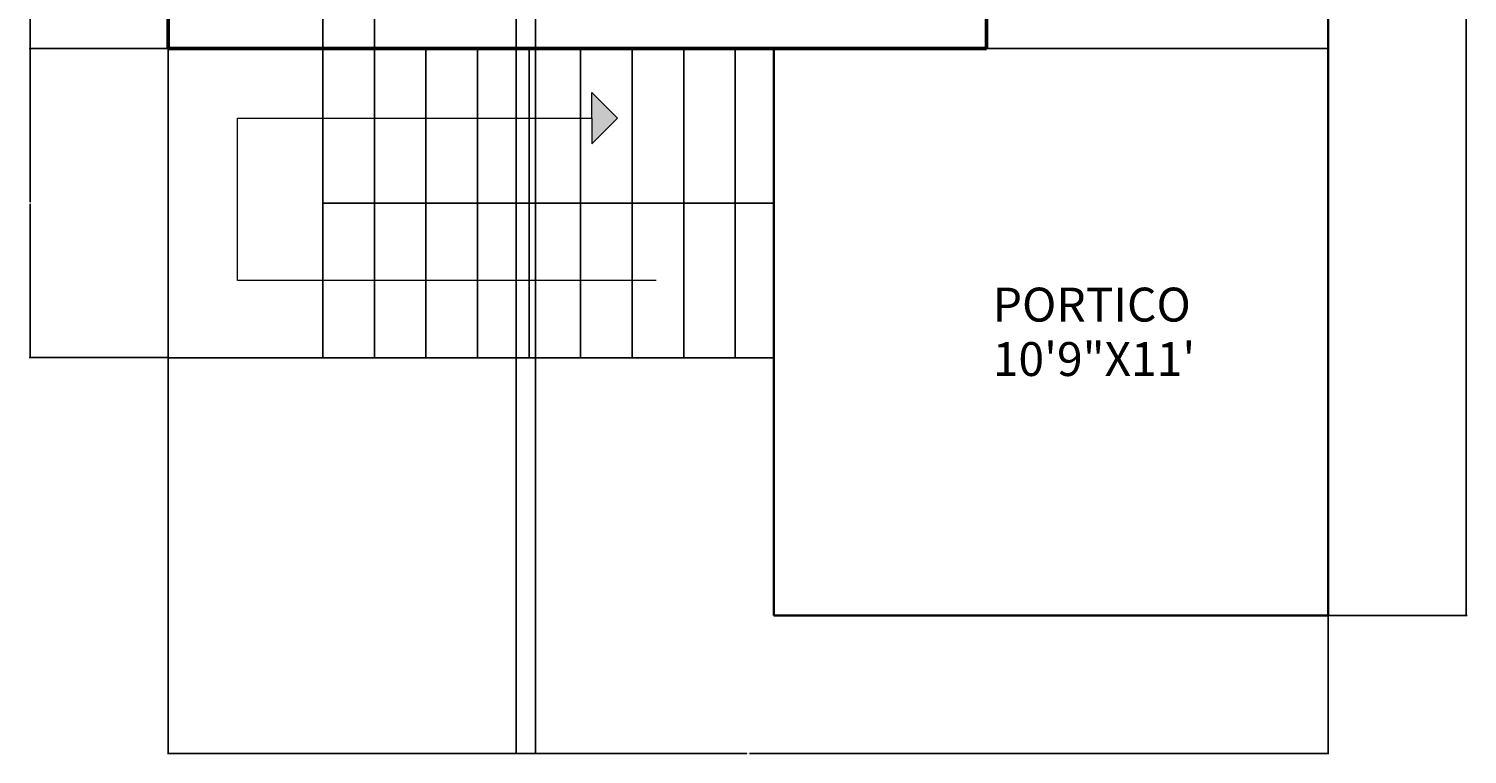
# Model space of a CAD drawing. Units: feet. Extents: x 1657 to 2001, y 1678 to 2367.
# Tile 1 of 4: x 1666 to 2001, y 1678 to 1847. Entities that reach past the tile are written whole.
import ezdxf

# ---------------------------------------------------------------- set-up
doc = ezdxf.new("R2010")
doc.units = ezdxf.units.FT
for name, color, linetype, lineweight in [('A-ANNO-DIMS', 2, 'Continuous', 18), ('A-ANNO-SYMB', 7, 'Continuous', 18), ('A-AREA-IDEN', 7, 'Continuous', 25), ('A-FLOR', 7, 'Continuous', 35), ('A-FLOR-STRS', 7, 'Continuous', 25), ('A-WALL', 7, 'Continuous', 50)]:
    doc.layers.add(name, color=color, linetype=linetype, lineweight=lineweight)
doc.styles.get("Standard").update_dxf_attribs({"font": 'arial.ttf'})
doc.dimstyles.get("Standard").update_dxf_attribs({"dimtxt": 0.18, "dimasz": 0.18, "dimexe": 0.18, "dimexo": 0.0625, "dimgap": 0.09, "dimtad": 0, "dimtih": 1, "dimtoh": 1, "dimdec": 4, "dimzin": 0, "dimdsep": 46, "dimtxsty": 'Standard', "dimcen": 0.09, "dimadec": 0, "dimazin": 0, "dimtfac": 1, "dimtdec": 4, "dimtofl": 0, "dimtmove": 0, "dimatfit": 3, "dimfxl": 1, "dimtolj": 1, "dimtzin": 0, "dimarcsym": 0})

# ---------------------------------------------------------------- blocks, each defined once
blk = doc.blocks.new('*D34')
at = {"layer": 'A-ANNO-DIMS', "color": 0, "lineweight": -2, "transparency": 16777216}
for p, q in [((1698.28, 1770.24), (1698.28, 1677.97)), ((1968.28, 1710.24), (1968.28, 1677.97)), ((1698.46, 1678.15), (1832.99, 1678.15)), ((1968.1, 1678.15), (1833.57, 1678.15))]:
    blk.add_line(p, q, dxfattribs=at)
at = {"layer": 'A-ANNO-DIMS', "color": 0, "transparency": 16777216}
for points in [[(1698.46, 1678.18), (1698.46, 1678.12), (1698.28, 1678.15)], [(1968.1, 1678.18), (1968.1, 1678.12), (1968.28, 1678.15)]]:
    blk.add_solid(points, dxfattribs=at)
at = {"layer": 'Defpoints', "color": 0, "transparency": 16777216}
for p in [(1698.28, 1770.3), (1968.28, 1710.3), (1968.28, 1678.15)]:
    blk.add_point(p, dxfattribs=at)
at = {"layer": 'A-ANNO-DIMS', "color": 0, "transparency": 16777216, "insert": (1833.28, 1678.15), "char_height": 0.18, "attachment_point": 5}
blk.add_mtext('\\A1;270', dxfattribs=at)
blk = doc.blocks.new('*D35')
at = {"layer": 'A-ANNO-DIMS', "color": 0, "lineweight": -2, "transparency": 16777216}
for p, q in [((1968.35, 2334.3), (2000.61, 2334.3)), ((2000.43, 2334.12), (2000.43, 2022.48)), ((2000.43, 1710.48), (2000.43, 2022.12)), ((1968.35, 1710.3), (2000.61, 1710.3))]:
    blk.add_line(p, q, dxfattribs=at)
at = {"layer": 'A-ANNO-DIMS', "color": 0, "transparency": 16777216}
for points in [[(2000.4, 2334.12), (2000.46, 2334.12), (2000.43, 2334.3)], [(2000.4, 1710.48), (2000.46, 1710.48), (2000.43, 1710.3)]]:
    blk.add_solid(points, dxfattribs=at)
at = {"layer": 'Defpoints', "color": 0, "transparency": 16777216}
for p in [(1968.28, 2334.3), (2000.43, 2334.3), (1968.28, 1710.3)]:
    blk.add_point(p, dxfattribs=at)
at = {"layer": 'A-ANNO-DIMS', "color": 0, "transparency": 16777216, "insert": (2000.43, 2022.3), "char_height": 0.18, "attachment_point": 5}
blk.add_mtext('\\A1;624', dxfattribs=at)
blk = doc.blocks.new('*D36')
at = {"layer": 'A-ANNO-DIMS', "color": 0, "lineweight": -2, "transparency": 16777216}
for p, q in [((1698.22, 1842.3), (1665.95, 1842.3)), ((1666.13, 1842.12), (1666.13, 1806.48)), ((1666.13, 1770.48), (1666.13, 1806.12)), ((1698.22, 1770.3), (1665.95, 1770.3))]:
    blk.add_line(p, q, dxfattribs=at)
at = {"layer": 'A-ANNO-DIMS', "color": 0, "transparency": 16777216}
for points in [[(1666.1, 1842.12), (1666.16, 1842.12), (1666.13, 1842.3)], [(1666.1, 1770.48), (1666.16, 1770.48), (1666.13, 1770.3)]]:
    blk.add_solid(points, dxfattribs=at)
at = {"layer": 'Defpoints', "color": 0, "transparency": 16777216}
for p in [(1666.13, 1842.3), (1698.28, 1842.3), (1698.28, 1770.3)]:
    blk.add_point(p, dxfattribs=at)
at = {"layer": 'A-ANNO-DIMS', "color": 0, "transparency": 16777216, "insert": (1666.13, 1806.3), "char_height": 0.18, "attachment_point": 5}
blk.add_mtext('\\A1;72', dxfattribs=at)
blk = doc.blocks.new('*D37')
at = {"layer": 'A-ANNO-DIMS', "color": 0, "lineweight": -2, "transparency": 16777216}
for p, q in [((1734.28, 1770.36), (1734.28, 2366.63)), ((1734.46, 2366.45), (1740.08, 2366.45)), ((1746.1, 2366.45), (1740.49, 2366.45)), ((1746.28, 1770.36), (1746.28, 2366.63))]:
    blk.add_line(p, q, dxfattribs=at)
at = {"layer": 'A-ANNO-DIMS', "color": 0, "transparency": 16777216}
for points in [[(1734.46, 2366.48), (1734.46, 2366.42), (1734.28, 2366.45)], [(1746.1, 2366.48), (1746.1, 2366.42), (1746.28, 2366.45)]]:
    blk.add_solid(points, dxfattribs=at)
at = {"layer": 'Defpoints', "color": 0, "transparency": 16777216}
for p in [(1746.28, 2366.45), (1734.28, 1770.3), (1746.28, 1770.3)]:
    blk.add_point(p, dxfattribs=at)
at = {"layer": 'A-ANNO-DIMS', "color": 0, "transparency": 16777216, "insert": (1740.28, 2366.45), "char_height": 0.18, "attachment_point": 5}
blk.add_mtext('\\A1;12', dxfattribs=at)
blk = doc.blocks.new('*D38')
at = {"layer": 'A-ANNO-DIMS', "color": 0, "lineweight": -2, "transparency": 16777216}
for p, q in [((1698.28, 1770.36), (1698.28, 2366.63)), ((1698.46, 2366.45), (1716.07, 2366.45)), ((1734.1, 2366.45), (1716.5, 2366.45)), ((1734.28, 1770.36), (1734.28, 2366.63))]:
    blk.add_line(p, q, dxfattribs=at)
at = {"layer": 'A-ANNO-DIMS', "color": 0, "transparency": 16777216}
for points in [[(1698.46, 2366.48), (1698.46, 2366.42), (1698.28, 2366.45)], [(1734.1, 2366.48), (1734.1, 2366.42), (1734.28, 2366.45)]]:
    blk.add_solid(points, dxfattribs=at)
at = {"layer": 'Defpoints', "color": 0, "transparency": 16777216}
for p in [(1734.28, 2366.45), (1698.28, 1770.3), (1734.28, 1770.3)]:
    blk.add_point(p, dxfattribs=at)
at = {"layer": 'A-ANNO-DIMS', "color": 0, "transparency": 16777216, "insert": (1716.28, 2366.45), "char_height": 0.18, "attachment_point": 5}
blk.add_mtext('\\A1;36', dxfattribs=at)
blk = doc.blocks.new('*D43')
at = {"layer": 'A-ANNO-DIMS', "color": 0, "lineweight": -2, "transparency": 16777216}
for p, q in [((1698.22, 1903.34), (1665.95, 1903.34)), ((1666.13, 1903.16), (1666.13, 1873)), ((1666.13, 1842.48), (1666.13, 1872.64)), ((1698.22, 1842.3), (1665.95, 1842.3))]:
    blk.add_line(p, q, dxfattribs=at)
at = {"layer": 'A-ANNO-DIMS', "color": 0, "transparency": 16777216}
for points in [[(1666.1, 1903.16), (1666.16, 1903.16), (1666.13, 1903.34)], [(1666.1, 1842.48), (1666.16, 1842.48), (1666.13, 1842.3)]]:
    blk.add_solid(points, dxfattribs=at)
at = {"layer": 'Defpoints', "color": 0, "transparency": 16777216}
for p in [(1666.13, 1903.34), (1698.28, 1903.34), (1698.28, 1842.3)]:
    blk.add_point(p, dxfattribs=at)
at = {"layer": 'A-ANNO-DIMS', "color": 0, "transparency": 16777216, "insert": (1666.13, 1872.82), "char_height": 0.18, "attachment_point": 5}
blk.add_mtext('\\A1;61.04', dxfattribs=at)
blk = doc.blocks.new('*D53')
at = {"layer": 'A-ANNO-DIMS', "color": 0, "lineweight": -2, "transparency": 16777216}
for p, q in [((1779.28, 1983.24), (1779.28, 1677.97)), ((1783.78, 1983.24), (1783.78, 1677.97)), ((1779.46, 1678.15), (1781.28, 1678.15)), ((1783.6, 1678.15), (1781.79, 1678.15))]:
    blk.add_line(p, q, dxfattribs=at)
at = {"layer": 'A-ANNO-DIMS', "color": 0, "transparency": 16777216}
for points in [[(1779.46, 1678.18), (1779.46, 1678.12), (1779.28, 1678.15)], [(1783.6, 1678.18), (1783.6, 1678.12), (1783.78, 1678.15)]]:
    blk.add_solid(points, dxfattribs=at)
at = {"layer": 'Defpoints', "color": 0, "transparency": 16777216}
for p in [(1779.28, 1983.3), (1783.78, 1983.3), (1783.78, 1678.15)]:
    blk.add_point(p, dxfattribs=at)
at = {"layer": 'A-ANNO-DIMS', "color": 0, "transparency": 16777216, "insert": (1781.53, 1678.15), "char_height": 0.18, "attachment_point": 5}
blk.add_mtext('\\A1;4.5', dxfattribs=at)

msp = doc.modelspace()

# ---------------------------------------------------------------- hatches: boundary and pattern name
at = {"layer": 'A-ANNO-SYMB'}
h = msp.add_hatch(color=256, dxfattribs=at)
h.dxf.hatch_style = 1
h.paths.add_polyline_path([(1802.875, 1826.0659), (1796.875, 1832.0659), (1796.875, 1826.0659), (1796.875, 1820.0659)])

# ---------------------------------------------------------------- linework, layer by layer
for p, q in [((1796.875, 1826.0659), (1796.875, 1832.0659)), ((1796.875, 1832.0659), (1802.875, 1826.0659)), ((1714.4003, 1788.2557), (1714.4003, 1826.0659)), ((1714.4003, 1826.0659), (1796.875, 1826.0659)), ((1796.875, 1826.0659), (1796.875, 1820.0659)), ((1802.875, 1826.0659), (1796.875, 1820.0659)), ((1811.8591, 1788.2557), (1714.4003, 1788.2557))]:
    msp.add_line(p, q, dxfattribs=at)
at = {"layer": 'A-FLOR'}
for p, q in [((1968.2848, 1842.2977), (1968.2848, 1983.2977)), ((1839.2848, 1710.2977), (1839.2848, 1842.2977)), ((1968.2848, 1842.2977), (1968.2848, 1710.2977)), ((1968.2848, 1710.2977), (1839.2848, 1710.2977))]:
    msp.add_line(p, q, dxfattribs=at)
at = {"layer": 'A-FLOR-STRS'}
for p, q in [((1698.2848, 1842.2977), (1698.2848, 1770.2977)), ((1734.2848, 1842.2977), (1734.2848, 1770.2977)), ((1746.2848, 1842.2977), (1746.2848, 1770.2977)), ((1758.2848, 1842.2977), (1758.2848, 1770.2977)), ((1770.2848, 1842.2977), (1770.2848, 1770.2977)), ((1782.2848, 1842.2977), (1782.2848, 1770.2977)), ((1794.2848, 1842.2977), (1794.2848, 1770.2977)), ((1806.2848, 1842.2977), (1806.2848, 1770.2977)), ((1818.2848, 1842.2977), (1818.2848, 1770.2977)), ((1830.2848, 1842.2977), (1830.2848, 1770.2977)), ((1888.7848, 1842.2977), (1968.2848, 1842.2977)), ((1734.2848, 1806.2977), (1839.2848, 1806.2977)), ((1698.2848, 1770.2977), (1839.2848, 1770.2977))]:
    msp.add_line(p, q, dxfattribs=at)
at = {"layer": 'A-WALL'}
for p, q in [((1698.2848, 2334.2977), (1698.2848, 1842.2977)), ((1698.2848, 1983.2977), (1698.2848, 1842.2977)), ((1888.7848, 1851.2977), (1888.7848, 1842.2977)), ((1698.2848, 1842.2977), (1888.7848, 1842.2977)), ((1783.7848, 1842.2977), (1888.7848, 1842.2977))]:
    msp.add_line(p, q, dxfattribs=at)

# ---------------------------------------------------------------- texts
at = {"layer": 'A-AREA-IDEN'}
for s, p in [('PORTICO', (1890.2079, 1778.7097)), ('10\'9"X11\'', (1890.2079, 1766.0345))]:
    msp.add_text(s, height=7.89038, dxfattribs=at).set_placement(p)

# ---------------------------------------------------------------- dimensions: what is measured, and where the dimension line sits
at = {"layer": 'A-ANNO-DIMS'}
for base, p1, p2, override, picture, middle in [((1734.2848, 2366.4477), (1698.2848, 1770.2977), (1734.2848, 1770.2977), {"dimdec": 0, "dimlfac": 1, "dimrnd": 0, "dimzin": 0, "dimdsep": 46, "dimlunit": 2}, '*D38', (1716.2848, 2366.4477)), ((1746.2848, 2366.4477), (1734.2848, 1770.2977), (1746.2848, 1770.2977), {"dimdec": 0, "dimlfac": 1, "dimrnd": 0, "dimzin": 0, "dimdsep": 46, "dimlunit": 2}, '*D37', (1740.2848, 2366.4477)), ((1783.7848, 1678.1477), (1779.2848, 1983.2977), (1783.7848, 1983.2977), {"dimdec": 1, "dimlfac": 1, "dimrnd": 0, "dimzin": 0, "dimdsep": 46, "dimlunit": 2}, '*D53', (1781.5348, 1678.1477)), ((1968.2848, 1678.1477), (1698.2848, 1770.2977), (1968.2848, 1710.2977), {"dimdec": 0, "dimlfac": 1, "dimrnd": 0, "dimzin": 0, "dimdsep": 46, "dimlunit": 2}, '*D34', (1833.2848, 1678.1477))]:
    dim = msp.add_linear_dim(base=base, p1=p1, p2=p2, dimstyle='Standard', override=override, dxfattribs=at)
    dim.commit()
    dim.dimension.update_dxf_attribs({"geometry": picture, "text_midpoint": middle})
for base, p1, p2, override, picture, middle in [((2000.4348, 2334.2977), (1968.2848, 1710.2977), (1968.2848, 2334.2977), {"dimdec": 0, "dimlfac": 1, "dimrnd": 0, "dimzin": 0, "dimdsep": 46, "dimlunit": 2}, '*D35', (2000.4348, 2022.2977)), ((1666.1348, 1903.3405), (1698.2848, 1842.2977), (1698.2848, 1903.3405), {"dimdec": 2, "dimlfac": 1, "dimrnd": 0, "dimzin": 0, "dimdsep": 46, "dimlunit": 2}, '*D43', (1666.1348, 1872.8191)), ((1666.1348, 1842.2977), (1698.2848, 1770.2977), (1698.2848, 1842.2977), {"dimdec": 0, "dimlfac": 1, "dimrnd": 0, "dimzin": 0, "dimdsep": 46, "dimlunit": 2}, '*D36', (1666.1348, 1806.2977))]:
    dim = msp.add_linear_dim(base=base, p1=p1, p2=p2, angle=90, dimstyle='Standard', override=override, dxfattribs=at)
    dim.commit()
    dim.dimension.update_dxf_attribs({"geometry": picture, "text_midpoint": middle})

doc.saveas('drawing.dxf')
